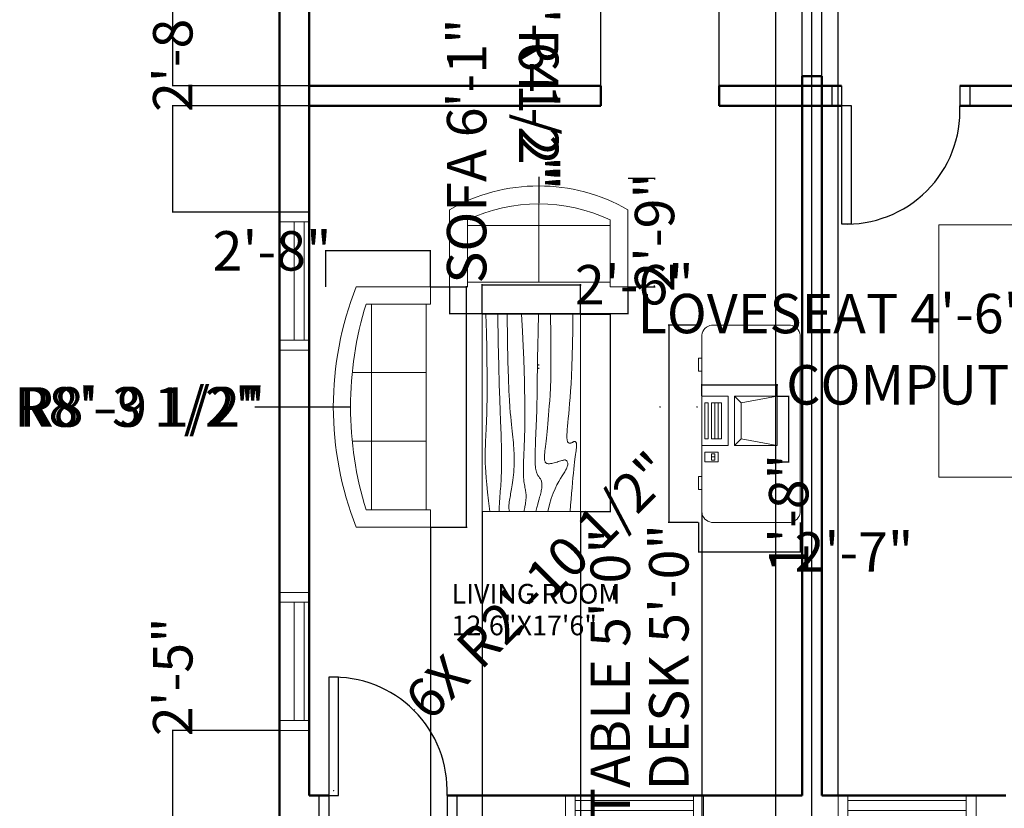
# Model space of a CAD drawing. Units: inches. Extents: x -51 to 1118, y -44 to 791.
# Tile 2 of 8: x -51 to 249, y 104 to 344. Entities that reach past the tile are written whole.
import ezdxf

# ---------------------------------------------------------------- set-up
doc = ezdxf.new("R2010")
doc.units = ezdxf.units.IN
doc.header["$MEASUREMENT"] = 0
for name, color, linetype, lineweight in [('A-ANNO-DIMS', 2, 'Continuous', 18), ('A-AREA-IDEN', 7, 'Continuous', 18), ('A-DOOR', 3, 'Continuous', 25), ('A-EQPM', 9, 'Continuous', 18), ('A-FURN', 8, 'Continuous', 18), ('A-GLAZ', 4, 'Continuous', 18), ('A-WALL', 7, 'Continuous', 50)]:
    doc.layers.add(name, color=color, linetype=linetype, lineweight=lineweight)
doc.styles.get("Standard").update_dxf_attribs({"font": 'arial.ttf'})
doc.dimstyles.get("Standard").update_dxf_attribs({"dimtxt": 12, "dimasz": 0.18, "dimexe": 0.18, "dimexo": 0.0625, "dimgap": 0.09, "dimtad": 0, "dimdec": 1, "dimzin": 0, "dimdsep": 46, "dimlunit": 3, "dimtxsty": 'Standard', "dimcen": 0.09, "dimadec": 0, "dimazin": 0, "dimtfac": 1, "dimtdec": 1, "dimtofl": 0, "dimtmove": 0, "dimatfit": 3, "dimfxl": 1, "dimtolj": 1, "dimtzin": 0, "dimarcsym": 0})

# ---------------------------------------------------------------- blocks, each defined once
blk = doc.blocks.new('Table - Rectangular Woodgrain 60 x 30 in.')
for p, q in [((0, 0), (0, -30)), ((60, 0), (0, 0)), ((60, -30), (60, 0)), ((0, -30), (60, -30))]:
    blk.add_line(p, q)
for points in [[(0, -2.4), (4.8155, -2.418), (9.0302, -2.4688), (12.709, -2.5477), (15.9167, -2.65), (18.7181, -2.7711), (21.1781, -2.9063), (23.3616, -3.0508), (25.3333, -3.2), (27.1477, -3.3495), (28.8172, -3.4958), (30.3437, -3.636), (31.7291, -3.7667), (32.9756, -3.8849), (34.0849, -3.9875), (35.059, -4.0714), (35.9, -4.1334), (36.6114, -4.1711), (37.2041, -4.1854), (37.6906, -4.1779), (38.0833, -4.15), (38.3948, -4.1034), (38.6375, -4.0396), (38.8239, -3.9602), (38.9666, -3.8667), (39.0764, -3.7608), (39.1573, -3.6448), (39.2116, -3.521), (39.2416, -3.3917), (39.2498, -3.2593), (39.2385, -3.1261), (39.21, -2.9944), (39.1666, -2.8667), (39.111, -2.7447), (39.0468, -2.6281), (38.978, -2.5163), (38.9083, -2.4083), (38.8418, -2.3035), (38.7823, -2.201), (38.7337, -2.1001), (38.7, -2), (38.6844, -1.9003), (38.6875, -1.8021), (38.7094, -1.707), (38.75, -1.6167), (38.8094, -1.5326), (38.8875, -1.4563), (38.9844, -1.3893), (39.1, -1.3333), (39.2351, -1.2896), (39.3937, -1.2583), (39.5804, -1.2396), (39.8, -1.2333), (40.057, -1.2396), (40.3562, -1.2583), (40.7023, -1.2896), (41.1, -1.3333), (41.5547, -1.3895), (42.0755, -1.4573), (42.6721, -1.5361), (43.3542, -1.625), (44.1316, -1.7233), (45.014, -1.8302), (46.0114, -1.9449), (47.1333, -2.0667), (48.3862, -2.1947), (49.7625, -2.3281), (51.2513, -2.4663), (52.8416, -2.6083), (54.5226, -2.7535), (56.2833, -2.9011), (58.1127, -3.0501), (60, -3.2)], [(0, -9.2), (6.5759, -9.0858), (11.9385, -9.0365), (16.2527, -9.0418), (19.6833, -9.0917), (22.3952, -9.1759), (24.5531, -9.2844), (26.322, -9.4069), (27.8666, -9.5333), (29.3241, -9.6553), (30.7203, -9.7719), (32.0532, -9.8837), (33.3208, -9.9917), (34.5213, -10.0965), (35.6526, -10.199), (36.7128, -10.2999), (37.7, -10.4), (38.6129, -10.4996), (39.4531, -10.5969), (40.223, -10.6895), (40.925, -10.775), (41.5613, -10.8512), (42.1344, -10.9156), (42.6465, -10.966), (43.1, -11), (43.4976, -11.0158), (43.8437, -11.0136), (44.143, -10.9942), (44.4, -10.9583), (44.6195, -10.9069), (44.8062, -10.8406), (44.9648, -10.7603), (45.1, -10.6667), (45.2155, -10.5598), (45.3114, -10.4365), (45.3871, -10.2929), (45.4416, -10.125), (45.4743, -9.929), (45.4844, -9.7011), (45.4709, -9.4371), (45.4333, -9.1333), (45.3716, -8.7883), (45.2896, -8.4104), (45.1919, -8.0107), (45.0833, -7.6), (44.9685, -7.1893), (44.8521, -6.7896), (44.7388, -6.4117), (44.6333, -6.0667), (44.54, -5.7628), (44.4614, -5.4979), (44.4001, -5.2675), (44.3583, -5.0667), (44.3384, -4.8909), (44.3427, -4.7354), (44.3736, -4.5956), (44.4333, -4.4667), (44.5236, -4.3453), (44.6427, -4.2333), (44.7884, -4.1339), (44.9583, -4.05), (45.1501, -3.9849), (45.3614, -3.9417), (45.59, -3.9234), (45.8333, -3.9333), (46.0915, -3.9749), (46.3734, -4.0531), (46.6906, -4.1736), (47.0542, -4.3417), (47.4756, -4.5629), (47.9661, -4.8427), (48.5372, -5.1866), (49.2, -5.6), (49.9676, -6.0844), (50.8594, -6.625), (51.8965, -7.2031), (53.1, -7.8), (54.491, -8.3969), (56.0906, -8.975), (57.9199, -9.5156), (60, -10)], [(0, -12.8), (5.1847, -12.9322), (9.6213, -13.0323), (13.3963, -13.1059), (16.5958, -13.1583), (19.3063, -13.1952), (21.614, -13.2219), (23.6054, -13.2439), (25.3666, -13.2667), (26.9728, -13.2947), (28.4531, -13.3281), (29.8256, -13.3663), (31.1083, -13.4083), (32.3191, -13.4535), (33.476, -13.501), (34.597, -13.5501), (35.7, -13.6), (36.7984, -13.6497), (37.8875, -13.6979), (38.9578, -13.743), (40, -13.7833), (41.0047, -13.8174), (41.9625, -13.8438), (42.864, -13.8607), (43.7, -13.8667), (44.4631, -13.8604), (45.1552, -13.8417), (45.7801, -13.8104), (46.3416, -13.7667), (46.8439, -13.7104), (47.2906, -13.6417), (47.6858, -13.5604), (48.0333, -13.4667), (48.3375, -13.3608), (48.6042, -13.2448), (48.8396, -13.121), (49.05, -12.9917), (49.2417, -12.8593), (49.4208, -12.7261), (49.5937, -12.5944), (49.7667, -12.4667), (49.9452, -12.3451), (50.1323, -12.2313), (50.3303, -12.1268), (50.5416, -12.0333), (50.7686, -11.9524), (51.0135, -11.8854), (51.2788, -11.8341), (51.5666, -11.8), (51.8785, -11.7843), (52.2116, -11.7865), (52.562, -11.8059), (52.926, -11.8417), (53.2998, -11.8931), (53.6795, -11.9594), (54.0614, -12.0397), (54.4416, -12.1333), (54.8223, -12.2401), (55.2293, -12.3625), (55.6942, -12.5037), (56.2489, -12.6667), (56.9251, -12.8547), (57.7545, -13.0708), (58.7689, -13.3182), (60, -13.6)], [(0, -18), (5.124, -17.7273), (9.6609, -17.5057), (13.6705, -17.3303), (17.2125, -17.1958), (20.3467, -17.0973), (23.1328, -17.0297), (25.6307, -16.9878), (27.9, -16.9667), (29.9928, -16.9617), (31.9302, -16.9703), (33.7254, -16.9907), (35.3917, -17.0208), (36.9423, -17.0588), (38.3906, -17.1026), (39.7499, -17.1503), (41.0333, -17.2), (42.2519, -17.2496), (43.4073, -17.2969), (44.4986, -17.3395), (45.525, -17.375), (46.4858, -17.4012), (47.3802, -17.4156), (48.2074, -17.416), (48.9667, -17.4), (49.6583, -17.3662), (50.2872, -17.3167), (50.8595, -17.2547), (51.3812, -17.1833), (51.8584, -17.1057), (52.2971, -17.025), (52.7034, -16.9443), (53.0833, -16.8667), (53.443, -16.7951), (53.789, -16.7313), (54.128, -16.6768), (54.4666, -16.6334), (54.8115, -16.6024), (55.1693, -16.5854), (55.5465, -16.5841), (55.95, -16.6), (56.3828, -16.6337), (56.8346, -16.6823), (57.2915, -16.7418), (57.7396, -16.8084), (58.165, -16.878), (58.5539, -16.9469), (58.8924, -17.0111), (59.1666, -17.0667), (59.3679, -17.1107), (59.5078, -17.1438), (59.6032, -17.1675), (59.6708, -17.1833), (59.7275, -17.193), (59.7901, -17.1979), (59.8753, -17.1998), (60, -17.2)], [(0, -22.4), (8.0098, -22.2501), (14.4094, -22.1011), (19.4168, -21.9535), (23.25, -21.8083), (26.1269, -21.6663), (28.2656, -21.5281), (29.884, -21.3947), (31.2, -21.2667), (32.3967, -21.1448), (33.5172, -21.0292), (34.5697, -20.9198), (35.5625, -20.8167), (36.5037, -20.7198), (37.4015, -20.6292), (38.2642, -20.5448), (39.1, -20.4667), (39.9164, -20.3951), (40.7187, -20.3313), (41.5117, -20.2768), (42.3, -20.2333), (43.0883, -20.2024), (43.8812, -20.1854), (44.6836, -20.1841), (45.5, -20.2), (46.3328, -20.234), (47.1747, -20.2844), (48.0163, -20.3488), (48.8479, -20.425), (49.66, -20.5106), (50.4429, -20.6031), (51.1872, -20.7004), (51.8833, -20.8), (52.5246, -20.8999), (53.1166, -20.9995), (53.6681, -21.0983), (54.1875, -21.1958), (54.6834, -21.2919), (55.1646, -21.3859), (55.6394, -21.4777), (56.1167, -21.5667), (56.6028, -21.6515), (57.0961, -21.7266), (57.5929, -21.7852), (58.0896, -21.8208), (58.5823, -21.8268), (59.0674, -21.7964), (59.5412, -21.723), (60, -21.6)], [(0, -25.2), (8.6355, -25.0504), (15.7026, -24.9031), (21.4049, -24.7606), (25.9458, -24.625), (29.529, -24.4988), (32.3578, -24.3844), (34.6359, -24.284), (36.5667, -24.2), (38.3213, -24.1341), (39.9417, -24.0854), (41.437, -24.0523), (42.8167, -24.0333), (44.0901, -24.0268), (45.2667, -24.0313), (46.3557, -24.0451), (47.3667, -24.0667), (48.309, -24.0947), (49.1928, -24.1287), (50.0284, -24.168), (50.826, -24.2125), (51.5959, -24.2617), (52.3483, -24.3151), (53.0935, -24.3725), (53.8417, -24.4334), (54.6009, -24.497), (55.3699, -24.561), (56.1454, -24.6226), (56.9239, -24.6792), (57.7021, -24.7279), (58.4764, -24.7662), (59.2435, -24.7911), (60, -24.8)], [(0, -28.8), (5.6867, -28.6681), (10.45, -28.5698), (14.407, -28.5012), (17.675, -28.4584), (20.3711, -28.4374), (22.6125, -28.4344), (24.5164, -28.4455), (26.2, -28.4667), (27.762, -28.4947), (29.2276, -28.5281), (30.6033, -28.5663), (31.8958, -28.6084), (33.1118, -28.6535), (34.2578, -28.7011), (35.3405, -28.7501), (36.3666, -28.8), (37.3443, -28.8497), (38.288, -28.8974), (39.2137, -28.9412), (40.1375, -28.9792), (41.0753, -29.0093), (42.0432, -29.0297), (43.0572, -29.0384), (44.1333, -29.0333), (45.2936, -29.0114), (46.5843, -28.9641), (48.0579, -28.8816), (49.7666, -28.7542), (51.7629, -28.5721), (54.0989, -28.3255), (56.8272, -28.0048), (60, -27.6)]]:
    blk.add_lwpolyline(points)
blk = doc.blocks.new('Computer Terminal')
for p, q in [((-10, 11.5), (5, 11.5)), ((-8, 0.5), (-10, 11.5)), ((-10, -1.5), (-10, 11.5)), ((5, 11.5), (3, 0.5)), ((5, 11.5), (5, -1.5)), ((-10, -1.5), (-8, 0.5)), ((3, 0.5), (-8, 0.5)), ((3, 0.5), (5, -1.5)), ((5, -1.5), (-10, -1.5)), ((-10, -11.5), (-10, -3.5)), ((-10, -3.5), (5, -3.5)), ((-8, -5.5), (-8, -8.5)), ((3, -5.5), (-8, -5.5)), ((3, -8.5), (3, -5.5)), ((5, -3.5), (5, -11.5)), ((3, -6.5), (-8, -6.5)), ((-8, -7.5), (3, -7.5)), ((-8, -8.5), (3, -8.5)), ((10, -6.5), (7, -6.5)), ((7, -6.5), (7, -10.5)), ((9.5, -7.5), (7.5, -7.5)), ((7.5, -7.5), (7.5, -8.5)), ((7.5, -8.5), (9.5, -8.5)), ((8.5, -7.5), (8.5, -8.5)), ((9.5, -8.5), (9.5, -7.5)), ((10, -10.5), (10, -6.5)), ((5, -11.5), (-10, -11.5)), ((-8, -9.5), (-8, -10.5)), ((3, -9.5), (-8, -9.5)), ((-8, -10.5), (3, -10.5)), ((3, -10.5), (3, -9.5)), ((7, -10.5), (10, -10.5))]:
    blk.add_line(p, q)
blk = doc.blocks.new('Desk - 30 x 60 in.')
for p, q in [((-26.999995, 0), (26.999995, 0)), ((-29.999995, -27), (-29.999995, -3)), ((29.999995, -3), (29.999995, -27)), ((26.999995, -30), (-26.999995, -30)), ((-20.000005, -30), (-20.000005, -31)), ((-20.000005, -31), (-16.000005, -31)), ((-16.000005, -31), (-16.000005, -30)), ((15.999995, -31), (15.999995, -30)), ((19.999995, -31), (15.999995, -31)), ((19.999995, -30), (19.999995, -31))]:
    blk.add_line(p, q)
for centre, start, end in [((-26.499995, -3.5), 98.1301, 171.8699), ((26.499995, -3.5), 8.130102, 81.8699), ((-26.499995, -26.5), 188.1301, 261.8699), ((26.499995, -26.5), 278.1301, 351.8699)]:
    blk.add_arc(centre, 3.535534, start, end)
blk = doc.blocks.new('Bed - Queen')
for p, q in [((0, -80.00003), (0, 0)), ((0, 0), (59.99999, 0)), ((59.99999, 0), (59.99999, -80.00003)), ((7.99999, -1.2), (28.79998, -1.2)), ((7.99999, -14.4), (7.99999, -1.2)), ((28.79998, -1.2), (28.79998, -14.4)), ((31.19999, -1.2), (51.99999, -1.2)), ((31.19999, -14.4), (31.19999, -1.2)), ((51.99999, -1.2), (51.99999, -16.4)), ((0, -14.4), (44.8, -14.4)), ((59.99999, -29.6), (44.8, -14.4)), ((44.8, -14.4), (44.8, -29.6)), ((44.8, -16.8), (0, -16.8)), ((51.99999, -16.4), (46.79936, -16.4)), ((44.8, -29.6), (59.99999, -29.6)), ((59.99999, -80.00003), (0, -80.00003))]:
    blk.add_line(p, q)
blk = doc.blocks.new('Sofa - Roundback Loveseat 5 ft.')
for p, q in [((0, -32.44198), (0, -5.99998)), ((-24, -33.99998), (-24, -11.46958)), ((24.00004, -33.99998), (24.00004, -11.46958)), ((-23.9998, -13.38178), (23.99986, -13.38178)), ((-24, -32.44198), (24.00004, -32.44198))]:
    blk.add_line(p, q)
for points in [[(-24, -33.99998), (-30, -33.99998), (-30, -7.99998)], [(30.00004, -7.99998), (30.00004, -33.99998), (24.00004, -33.99998)]]:
    blk.add_lwpolyline(points)
for centre, radius, start, end in [((0, -60.24998), 60.24998, 60.13715, 119.8628), ((0, -61.38438), 55.38444, 64.32083, 115.6792)]:
    blk.add_arc(centre, radius, start, end)
blk = doc.blocks.new('Sofa - Roundback 7 ft.')
for p, q in [((-12.00002, -32.4421), (-12.00003, -6.5971)), ((11.99997, -32.4421), (11.99998, -6.5971)), ((-36.000027, -34), (-36.000027, -11.4696)), ((-35.999844, -13.3819), (35.9998, -13.3819)), ((35.99998, -34), (35.99998, -11.4696)), ((-36.000027, -32.4421), (35.99998, -32.4421))]:
    blk.add_line(p, q)
for points in [[(-36.000027, -34), (-42.000027, -34), (-42.000027, -8)], [(41.99998, -8), (41.99998, -34), (35.99998, -34)]]:
    blk.add_lwpolyline(points)
for centre, radius, start, end in [((0, -114.25), 114.25, 68.43141, 111.5686), ((-0.00001, -127.1968), 121.1968, 72.72033, 107.2797)]:
    blk.add_arc(centre, radius, start, end)
blk = doc.blocks.new('WIN-36IN')
for p, q in [((9, 42), (0, 42)), ((9, 39), (0, 39)), ((0, 39), (0, 3)), ((4.5, 3), (4.5, 39)), ((7.5, 3), (7.5, 39)), ((9, 3), (9, 39)), ((0, 3), (9, 3)), ((0, 0), (9, 0))]:
    blk.add_line(p, q)
blk = doc.blocks.new('DOOR-36IN-FRAME-9IN')
for p, q in [((0, 36.03), (0, 45.03)), ((3, 36.03), (3, 45.03)), ((39, 36.03), (39, 45.03)), ((42, 36.03), (42, 45.03))]:
    blk.add_line(p, q)
blk.add_lwpolyline([(39, 36.03), (36, 36.03), (36, 0.03), (39, 0.03)], close=True)
blk.add_arc((37.5, 34.53), 34.53, 177.5104, 272.4896)
blk = doc.blocks.new('DOOR-36IN-FRAME-6IN')
for p, q in [((0, 42), (6, 42)), ((0, 39), (6, 39)), ((0, 3), (6, 3)), ((0, 0), (6, 0))]:
    blk.add_line(p, q)
blk.add_lwpolyline([(6, 3), (42, 3), (42, 6), (6, 6)], close=True)
blk.add_arc((7.5, 4.5), 34.53, 357.5104, 92.4896)
blk = doc.blocks.new('*D28')
at = {"layer": 'A-ANNO-DIMS', "color": 0, "lineweight": -2, "transparency": 16777216}
for p, q in [((119.72, 254.44), (128.83, 254.44)), ((128.65, 254.26), (128.65, 194.62)), ((119.72, 194.44), (128.83, 194.44)), ((128.65, 194.44), (128.65, 194.26))]:
    blk.add_line(p, q, dxfattribs=at)
at = {"layer": 'A-ANNO-DIMS', "color": 0, "transparency": 16777216}
for points in [[(128.62, 254.26), (128.68, 254.26), (128.65, 254.44)], [(128.62, 194.62), (128.68, 194.62), (128.65, 194.44)]]:
    blk.add_solid(points, dxfattribs=at)
at = {"layer": 'Defpoints', "color": 0, "transparency": 16777216}
for p in [(119.65, 254.44), (119.65, 194.44), (128.65, 194.44)]:
    blk.add_point(p, dxfattribs=at)
at = {"layer": 'A-ANNO-DIMS', "color": 0, "transparency": 16777216, "insert": (128.65, 113.08), "char_height": 12, "attachment_point": 5, "rotation": 90}
blk.add_mtext('\\A1;COFFEE TABLE 5\'-0"', dxfattribs=at)
blk = doc.blocks.new('*D29')
at = {"layer": 'A-ANNO-DIMS', "color": 0, "lineweight": -2, "transparency": 16777216}
for p, q in [((89.65, 254.5), (89.65, 263.62)), ((119.65, 254.5), (119.65, 263.62)), ((89.83, 263.44), (119.47, 263.44)), ((119.65, 263.44), (119.83, 263.44))]:
    blk.add_line(p, q, dxfattribs=at)
at = {"layer": 'A-ANNO-DIMS', "color": 0, "transparency": 16777216}
for points in [[(89.83, 263.47), (89.83, 263.41), (89.65, 263.44)], [(119.47, 263.47), (119.47, 263.41), (119.65, 263.44)]]:
    blk.add_solid(points, dxfattribs=at)
at = {"layer": 'Defpoints', "color": 0, "transparency": 16777216}
for p in [(119.65, 263.44), (89.65, 254.44), (119.65, 254.44)]:
    blk.add_point(p, dxfattribs=at)
at = {"layer": 'A-ANNO-DIMS', "color": 0, "transparency": 16777216, "insert": (135.98, 263.44), "char_height": 12, "attachment_point": 5}
blk.add_mtext('\\A1;2\'-6"', dxfattribs=at)
blk = doc.blocks.new('*D30')
at = {"layer": 'A-ANNO-DIMS', "color": 0, "lineweight": -2, "transparency": 16777216}
for p, q in [((156.48, 229.58), (156.48, 233.14)), ((156.66, 232.96), (179.3, 232.96)), ((179.48, 229.58), (179.48, 233.14)), ((179.48, 232.96), (179.66, 232.96))]:
    blk.add_line(p, q, dxfattribs=at)
at = {"layer": 'A-ANNO-DIMS', "color": 0, "transparency": 16777216}
for points in [[(156.66, 232.99), (156.66, 232.93), (156.48, 232.96)], [(179.3, 232.99), (179.3, 232.93), (179.48, 232.96)]]:
    blk.add_solid(points, dxfattribs=at)
at = {"layer": 'Defpoints', "color": 0, "transparency": 16777216}
for p in [(179.48, 232.96), (156.48, 229.51), (179.48, 229.51)]:
    blk.add_point(p, dxfattribs=at)
at = {"layer": 'A-ANNO-DIMS', "color": 0, "transparency": 16777216, "insert": (250.58, 232.96), "char_height": 12, "attachment_point": 5}
blk.add_mtext('\\A1;COMPUTER 1\'-11"', dxfattribs=at)
blk = doc.blocks.new('*D31')
at = {"layer": 'A-ANNO-DIMS', "color": 0, "lineweight": -2, "transparency": 16777216}
for p, q in [((179.54, 229.51), (183.11, 229.51)), ((182.93, 229.33), (182.93, 209.69)), ((179.54, 209.51), (183.11, 209.51)), ((182.93, 209.51), (182.93, 209.33))]:
    blk.add_line(p, q, dxfattribs=at)
at = {"layer": 'A-ANNO-DIMS', "color": 0, "transparency": 16777216}
for points in [[(182.9, 229.33), (182.96, 229.33), (182.93, 229.51)], [(182.9, 209.69), (182.96, 209.69), (182.93, 209.51)]]:
    blk.add_solid(points, dxfattribs=at)
at = {"layer": 'Defpoints', "color": 0, "transparency": 16777216}
for p in [(179.48, 229.51), (179.48, 209.51), (182.93, 209.51)]:
    blk.add_point(p, dxfattribs=at)
at = {"layer": 'A-ANNO-DIMS', "color": 0, "transparency": 16777216, "insert": (182.93, 193.86), "char_height": 12, "attachment_point": 5, "rotation": 90}
blk.add_mtext('\\A1;1\'-8"', dxfattribs=at)
blk = doc.blocks.new('*D32')
at = {"layer": 'A-ANNO-DIMS', "color": 0, "lineweight": -2, "transparency": 16777216}
for p, q in [((155.41, 251.11), (146.3, 251.11)), ((146.48, 250.93), (146.48, 191.29)), ((155.41, 191.11), (146.3, 191.11)), ((146.48, 191.11), (146.48, 190.93))]:
    blk.add_line(p, q, dxfattribs=at)
at = {"layer": 'A-ANNO-DIMS', "color": 0, "transparency": 16777216}
for points in [[(146.45, 250.93), (146.51, 250.93), (146.48, 251.11)], [(146.45, 191.29), (146.51, 191.29), (146.48, 191.11)]]:
    blk.add_solid(points, dxfattribs=at)
at = {"layer": 'Defpoints', "color": 0, "transparency": 16777216}
for p in [(155.48, 251.11), (146.48, 191.11), (155.48, 191.11)]:
    blk.add_point(p, dxfattribs=at)
at = {"layer": 'A-ANNO-DIMS', "color": 0, "transparency": 16777216, "insert": (146.48, 150.04), "char_height": 12, "attachment_point": 5, "rotation": 90}
blk.add_mtext('\\A1;DESK 5\'-0"', dxfattribs=at)
blk = doc.blocks.new('*D33')
at = {"layer": 'A-ANNO-DIMS', "color": 0, "lineweight": -2, "transparency": 16777216}
for p, q in [((155.48, 191.05), (155.48, 181.93)), ((186.48, 191.05), (186.48, 181.93)), ((155.66, 182.11), (186.3, 182.11)), ((186.48, 182.11), (186.66, 182.11))]:
    blk.add_line(p, q, dxfattribs=at)
at = {"layer": 'A-ANNO-DIMS', "color": 0, "transparency": 16777216}
for points in [[(155.66, 182.14), (155.66, 182.08), (155.48, 182.11)], [(186.3, 182.14), (186.3, 182.08), (186.48, 182.11)]]:
    blk.add_solid(points, dxfattribs=at)
at = {"layer": 'Defpoints', "color": 0, "transparency": 16777216}
for p in [(155.48, 191.11), (186.48, 191.11), (186.48, 182.11)]:
    blk.add_point(p, dxfattribs=at)
at = {"layer": 'A-ANNO-DIMS', "color": 0, "transparency": 16777216, "insert": (202.8, 182.11), "char_height": 12, "attachment_point": 5}
blk.add_mtext('\\A1;2\'-7"', dxfattribs=at)
blk = doc.blocks.new('*D36')
at = {"layer": 'A-ANNO-DIMS', "color": 0, "lineweight": -2, "transparency": 16777216}
for p, q in [((79.8, 262.73), (79.8, 254.48)), ((134, 262.73), (134, 254.48)), ((79.98, 254.66), (133.82, 254.66)), ((134, 254.66), (134.18, 254.66))]:
    blk.add_line(p, q, dxfattribs=at)
at = {"layer": 'A-ANNO-DIMS', "color": 0, "transparency": 16777216}
for points in [[(79.98, 254.69), (79.98, 254.63), (79.8, 254.66)], [(133.82, 254.69), (133.82, 254.63), (134, 254.66)]]:
    blk.add_solid(points, dxfattribs=at)
at = {"layer": 'Defpoints', "color": 0, "transparency": 16777216}
for p in [(79.8, 262.79), (134, 262.79), (134, 254.66)]:
    blk.add_point(p, dxfattribs=at)
at = {"layer": 'A-ANNO-DIMS', "color": 0, "transparency": 16777216, "insert": (196.54, 254.66), "char_height": 12, "attachment_point": 5}
blk.add_mtext('\\A1;LOVESEAT 4\'-6"', dxfattribs=at)
blk = doc.blocks.new('*D37')
at = {"layer": 'A-ANNO-DIMS', "color": 0, "lineweight": -2, "transparency": 16777216}
for p, q in [((134.06, 295.91), (142.31, 295.91)), ((142.13, 295.73), (142.13, 295.49)), ((134.06, 262.79), (142.31, 262.79)), ((142.13, 262.97), (142.13, 263.21))]:
    blk.add_line(p, q, dxfattribs=at)
at = {"layer": 'A-ANNO-DIMS', "color": 0, "transparency": 16777216}
for points in [[(142.1, 295.73), (142.16, 295.73), (142.13, 295.91)], [(142.1, 262.97), (142.16, 262.97), (142.13, 262.79)]]:
    blk.add_solid(points, dxfattribs=at)
at = {"layer": 'Defpoints', "color": 0, "transparency": 16777216}
for p in [(134, 295.91), (142.13, 295.91), (134, 262.79)]:
    blk.add_point(p, dxfattribs=at)
at = {"layer": 'A-ANNO-DIMS', "color": 0, "transparency": 16777216, "insert": (142.13, 279.35), "char_height": 12, "attachment_point": 5, "rotation": 90}
blk.add_mtext('\\A1;2\'-9"', dxfattribs=at)
blk = doc.blocks.new('*D38')
at = {"layer": 'A-ANNO-DIMS', "color": 0, "lineweight": -2, "transparency": 16777216}
for p, q in [((74.06, 262.79), (85.15, 262.79)), ((84.97, 262.79), (84.97, 262.97)), ((84.97, 189.87), (84.97, 262.61)), ((74.06, 189.69), (85.15, 189.69))]:
    blk.add_line(p, q, dxfattribs=at)
at = {"layer": 'A-ANNO-DIMS', "color": 0, "transparency": 16777216}
for points in [[(84.94, 262.61), (85, 262.61), (84.97, 262.79)], [(84.94, 189.87), (85, 189.87), (84.97, 189.69)]]:
    blk.add_solid(points, dxfattribs=at)
at = {"layer": 'Defpoints', "color": 0, "transparency": 16777216}
for p in [(74, 262.79), (84.97, 262.79), (74, 189.69)]:
    blk.add_point(p, dxfattribs=at)
at = {"layer": 'A-ANNO-DIMS', "color": 0, "transparency": 16777216, "insert": (84.97, 304.13), "char_height": 12, "attachment_point": 5, "rotation": 90}
blk.add_mtext('\\A1;SOFA 6\'-1"', dxfattribs=at)
blk = doc.blocks.new('*D39')
at = {"layer": 'A-ANNO-DIMS', "color": 0, "lineweight": -2, "transparency": 16777216}
for p, q in [((42.09, 273.75), (41.91, 273.75)), ((42.09, 262.85), (42.09, 273.93)), ((73.82, 273.75), (42.27, 273.75)), ((74, 262.85), (74, 273.93))]:
    blk.add_line(p, q, dxfattribs=at)
at = {"layer": 'A-ANNO-DIMS', "color": 0, "transparency": 16777216}
for points in [[(42.27, 273.78), (42.27, 273.72), (42.09, 273.75)], [(73.82, 273.78), (73.82, 273.72), (74, 273.75)]]:
    blk.add_solid(points, dxfattribs=at)
at = {"layer": 'Defpoints', "color": 0, "transparency": 16777216}
for p in [(42.09, 273.75), (42.09, 262.79), (74, 262.79)]:
    blk.add_point(p, dxfattribs=at)
at = {"layer": 'A-ANNO-DIMS', "color": 0, "transparency": 16777216, "insert": (25.77, 273.75), "char_height": 12, "attachment_point": 5}
blk.add_mtext('\\A1;2\'-8"', dxfattribs=at)
blk = doc.blocks.new('*D44')
at = {"layer": 'A-ANNO-DIMS', "color": 0, "lineweight": -2, "transparency": 16777216}
for p, q in [((27.96, 127.77), (-4.61, 127.77)), ((-4.43, 127.77), (-4.43, 127.95)), ((-4.43, 99.12), (-4.43, 127.59)), ((36.96, 98.94), (-4.61, 98.94))]:
    blk.add_line(p, q, dxfattribs=at)
at = {"layer": 'A-ANNO-DIMS', "color": 0, "transparency": 16777216}
for points in [[(-4.46, 127.59), (-4.4, 127.59), (-4.43, 127.77)], [(-4.46, 99.12), (-4.4, 99.12), (-4.43, 98.94)]]:
    blk.add_solid(points, dxfattribs=at)
at = {"layer": 'Defpoints', "color": 0, "transparency": 16777216}
for p in [(-4.43, 127.77), (28.02, 127.77), (37.02, 98.94)]:
    blk.add_point(p, dxfattribs=at)
at = {"layer": 'A-ANNO-DIMS', "color": 0, "transparency": 16777216, "insert": (-4.43, 144.09), "char_height": 12, "attachment_point": 5, "rotation": 90}
blk.add_mtext('\\A1;2\'-5"', dxfattribs=at)
blk = doc.blocks.new('*D45')
at = {"layer": 'A-ANNO-DIMS', "color": 0, "lineweight": -2, "transparency": 16777216}
for p, q in [((36.96, 317.94), (-4.61, 317.94)), ((-4.43, 317.94), (-4.43, 318.12)), ((-4.43, 285.72), (-4.43, 317.76)), ((36.96, 285.54), (-4.61, 285.54))]:
    blk.add_line(p, q, dxfattribs=at)
at = {"layer": 'A-ANNO-DIMS', "color": 0, "transparency": 16777216}
for points in [[(-4.46, 317.76), (-4.4, 317.76), (-4.43, 317.94)], [(-4.46, 285.72), (-4.4, 285.72), (-4.43, 285.54)]]:
    blk.add_solid(points, dxfattribs=at)
at = {"layer": 'Defpoints', "color": 0, "transparency": 16777216}
for p in [(-4.43, 317.94), (37.02, 317.94), (37.02, 285.54)]:
    blk.add_point(p, dxfattribs=at)
at = {"layer": 'A-ANNO-DIMS', "color": 0, "transparency": 16777216, "insert": (-4.43, 348.24), "char_height": 12, "attachment_point": 5, "rotation": 90}
blk.add_mtext('\\A1;2\'-8 1/2"', dxfattribs=at)
blk = doc.blocks.new('*D46')
at = {"layer": 'A-ANNO-DIMS', "color": 0, "lineweight": -2, "transparency": 16777216}
for p, q in [((36.96, 375.28), (-4.61, 375.28)), ((-4.43, 375.28), (-4.43, 375.46)), ((-4.43, 324.12), (-4.43, 375.1)), ((36.96, 323.94), (-4.61, 323.94))]:
    blk.add_line(p, q, dxfattribs=at)
at = {"layer": 'A-ANNO-DIMS', "color": 0, "transparency": 16777216}
for points in [[(-4.46, 375.1), (-4.4, 375.1), (-4.43, 375.28)], [(-4.46, 324.12), (-4.4, 324.12), (-4.43, 323.94)]]:
    blk.add_solid(points, dxfattribs=at)
at = {"layer": 'Defpoints', "color": 0, "transparency": 16777216}
for p in [(-4.43, 375.28), (37.02, 375.28), (37.02, 323.94)]:
    blk.add_point(p, dxfattribs=at)
at = {"layer": 'A-ANNO-DIMS', "color": 0, "transparency": 16777216, "insert": (-4.43, 405.72), "char_height": 12, "attachment_point": 5, "rotation": 90}
blk.add_mtext('\\A1;4\'-3 1/2"', dxfattribs=at)
blk = doc.blocks.new('*D55')
at = {"layer": 'A-ANNO-DIMS', "color": 0, "lineweight": -2, "transparency": 16777216}
for p, q in [((193.02, 108), (193.02, 638.57)), ((193.2, 638.39), (197.79, 638.39)), ((197.97, 108), (197.97, 638.57)), ((197.97, 638.39), (198.15, 638.39))]:
    blk.add_line(p, q, dxfattribs=at)
at = {"layer": 'A-ANNO-DIMS', "color": 0, "transparency": 16777216}
for points in [[(193.2, 638.42), (193.2, 638.36), (193.02, 638.39)], [(197.79, 638.42), (197.79, 638.36), (197.97, 638.39)]]:
    blk.add_solid(points, dxfattribs=at)
at = {"layer": 'Defpoints', "color": 0, "transparency": 16777216}
for p in [(197.97, 638.39), (193.02, 107.94), (197.97, 107.94)]:
    blk.add_point(p, dxfattribs=at)
at = {"layer": 'A-ANNO-DIMS', "color": 0, "transparency": 16777216, "insert": (214.19, 638.39), "char_height": 12, "attachment_point": 5}
blk.add_mtext('\\A1;0\'-5"', dxfattribs=at)
blk = doc.blocks.new('*D57')
at = {"layer": 'A-ANNO-DIMS', "color": 0, "lineweight": -2, "transparency": 16777216}
for p, q in [((179.02, 57), (179.02, 638.57)), ((179.2, 638.39), (189.84, 638.39)), ((190.02, 57), (190.02, 638.57)), ((190.02, 638.39), (190.2, 638.39))]:
    blk.add_line(p, q, dxfattribs=at)
at = {"layer": 'A-ANNO-DIMS', "color": 0, "transparency": 16777216}
for points in [[(179.2, 638.42), (179.2, 638.36), (179.02, 638.39)], [(189.84, 638.42), (189.84, 638.36), (190.02, 638.39)]]:
    blk.add_solid(points, dxfattribs=at)
at = {"layer": 'Defpoints', "color": 0, "transparency": 16777216}
for p in [(190.02, 638.39), (179.02, 56.94), (190.02, 56.94)]:
    blk.add_point(p, dxfattribs=at)
at = {"layer": 'A-ANNO-DIMS', "color": 0, "transparency": 16777216, "insert": (210.9, 638.39), "char_height": 12, "attachment_point": 5}
blk.add_mtext('\\A1;0\'-11"', dxfattribs=at)
blk = doc.blocks.new('*D59')
at = {"layer": 'A-ANNO-DIMS', "color": 0, "lineweight": -2, "transparency": 16777216}
for p, q in [((89.65, 194.38), (89.65, -26.69)), ((74, 189.63), (74, -26.69)), ((74.18, -26.51), (89.47, -26.51)), ((89.65, -26.51), (89.83, -26.51))]:
    blk.add_line(p, q, dxfattribs=at)
at = {"layer": 'A-ANNO-DIMS', "color": 0, "transparency": 16777216}
for points in [[(74.18, -26.48), (74.18, -26.54), (74, -26.51)], [(89.47, -26.48), (89.47, -26.54), (89.65, -26.51)]]:
    blk.add_solid(points, dxfattribs=at)
at = {"layer": 'Defpoints', "color": 0, "transparency": 16777216}
for p in [(89.65, 194.44), (74, 189.69), (89.65, -26.51)]:
    blk.add_point(p, dxfattribs=at)
at = {"layer": 'A-ANNO-DIMS', "color": 0, "transparency": 16777216, "insert": (119.29, -26.51), "char_height": 12, "attachment_point": 5}
blk.add_mtext('\\A1;1\'-3 1/2"', dxfattribs=at)
blk = doc.blocks.new('*D60')
at = {"layer": 'A-ANNO-DIMS', "color": 0, "lineweight": -2, "transparency": 16777216}
for p, q in [((119.65, 194.38), (119.65, -26.69)), ((156.48, 194.05), (156.48, -26.69)), ((119.83, -26.51), (122.03, -26.51)), ((156.3, -26.51), (154.1, -26.51))]:
    blk.add_line(p, q, dxfattribs=at)
at = {"layer": 'A-ANNO-DIMS', "color": 0, "transparency": 16777216}
for points in [[(119.83, -26.48), (119.83, -26.54), (119.65, -26.51)], [(156.3, -26.48), (156.3, -26.54), (156.48, -26.51)]]:
    blk.add_solid(points, dxfattribs=at)
at = {"layer": 'Defpoints', "color": 0, "transparency": 16777216}
for p in [(119.65, 194.44), (156.48, 194.11), (156.48, -26.51)]:
    blk.add_point(p, dxfattribs=at)
at = {"layer": 'A-ANNO-DIMS', "color": 0, "transparency": 16777216, "insert": (138.06, -26.51), "char_height": 12, "attachment_point": 5}
blk.add_mtext('\\A1;3\'-1"', dxfattribs=at)
blk = doc.blocks.new('*D61')
at = {"layer": 'A-ANNO-DIMS', "color": 0, "lineweight": -2, "transparency": 16777216}
for p, q in [((125.75, 324), (125.75, 638.57)), ((125.93, 638.39), (127.71, 638.39)), ((161.57, 638.39), (159.79, 638.39)), ((161.75, 324), (161.75, 638.57))]:
    blk.add_line(p, q, dxfattribs=at)
at = {"layer": 'A-ANNO-DIMS', "color": 0, "transparency": 16777216}
for points in [[(125.93, 638.42), (125.93, 638.36), (125.75, 638.39)], [(161.57, 638.42), (161.57, 638.36), (161.75, 638.39)]]:
    blk.add_solid(points, dxfattribs=at)
at = {"layer": 'Defpoints', "color": 0, "transparency": 16777216}
for p in [(161.75, 638.39), (125.75, 323.94), (161.75, 323.94)]:
    blk.add_point(p, dxfattribs=at)
at = {"layer": 'A-ANNO-DIMS', "color": 0, "transparency": 16777216, "insert": (143.75, 638.39), "char_height": 12, "attachment_point": 5}
blk.add_mtext('\\A1;3\'-0"', dxfattribs=at)
blk = doc.blocks.new('*D62')
at = {"layer": 'A-ANNO-DIMS', "color": 0, "lineweight": -2, "transparency": 16777216}
for p, q in [((161.75, 324), (161.75, 638.57)), ((161.93, 638.39), (186.84, 638.39)), ((187.02, 327), (187.02, 638.57)), ((187.02, 638.39), (187.2, 638.39))]:
    blk.add_line(p, q, dxfattribs=at)
at = {"layer": 'A-ANNO-DIMS', "color": 0, "transparency": 16777216}
for points in [[(161.93, 638.42), (161.93, 638.36), (161.75, 638.39)], [(186.84, 638.42), (186.84, 638.36), (187.02, 638.39)]]:
    blk.add_solid(points, dxfattribs=at)
at = {"layer": 'Defpoints', "color": 0, "transparency": 16777216}
for p in [(187.02, 638.39), (187.02, 326.94), (161.75, 323.94)]:
    blk.add_point(p, dxfattribs=at)
at = {"layer": 'A-ANNO-DIMS', "color": 0, "transparency": 16777216, "insert": (217.32, 638.39), "char_height": 12, "attachment_point": 5}
blk.add_mtext('\\A1;2\'-1 1/2"', dxfattribs=at)
blk = doc.blocks.new('*D67')
at = {"layer": 'A-ANNO-DIMS', "color": 0, "lineweight": -2, "transparency": 16777216}
for p, q in [((69.19, 134.11), (69.07, 133.99)), ((44.43, 109.44), (44.61, 109.44)), ((44.52, 109.35), (44.52, 109.53))]:
    blk.add_line(p, q, dxfattribs=at)
at = {"layer": 'A-ANNO-DIMS', "color": 0, "transparency": 16777216}
blk.add_solid([(69.05, 134.01), (69.09, 133.96), (68.94, 133.86)], dxfattribs=at)
at = {"layer": 'Defpoints', "color": 0, "transparency": 16777216}
for p in [(68.94, 133.86), (44.52, 109.44)]:
    blk.add_point(p, dxfattribs=at)
at = {"layer": 'A-ANNO-DIMS', "color": 0, "transparency": 16777216, "insert": (106.92, 171.84), "char_height": 12, "attachment_point": 5, "rotation": 45.0005}
blk.add_mtext('\\A1;6X R2\'-10 1/2"', dxfattribs=at)
blk = doc.blocks.new('*D68')
at = {"layer": 'A-ANNO-DIMS', "color": 0, "lineweight": -2, "transparency": 16777216}
for p, q in [((22.11, 226.24), (49.45, 226.24)), ((155.02, 226.24), (155.2, 226.24)), ((155.11, 226.15), (155.11, 226.33))]:
    blk.add_line(p, q, dxfattribs=at)
at = {"layer": 'A-ANNO-DIMS', "color": 0, "transparency": 16777216}
blk.add_solid([(49.45, 226.27), (49.45, 226.21), (49.63, 226.24)], dxfattribs=at)
at = {"layer": 'Defpoints', "color": 0, "transparency": 16777216}
for p in [(49.63, 226.24), (155.11, 226.24)]:
    blk.add_point(p, dxfattribs=at)
at = {"layer": 'A-ANNO-DIMS', "color": 0, "transparency": 16777216, "insert": (-13.65, 226.24), "char_height": 12, "attachment_point": 5, "rotation": 359.9999}
blk.add_mtext('\\A1;R8\'-9 1/2"', dxfattribs=at)
blk = doc.blocks.new('*D69')
at = {"layer": 'A-ANNO-DIMS', "color": 0, "lineweight": -2, "transparency": 16777216}
for p, q in [((20.52, 226.24), (44.23, 226.24)), ((143.75, 226.24), (143.93, 226.24)), ((143.84, 226.15), (143.84, 226.33))]:
    blk.add_line(p, q, dxfattribs=at)
at = {"layer": 'A-ANNO-DIMS', "color": 0, "transparency": 16777216}
blk.add_solid([(44.23, 226.27), (44.23, 226.21), (44.41, 226.24)], dxfattribs=at)
at = {"layer": 'Defpoints', "color": 0, "transparency": 16777216}
for p in [(44.41, 226.24), (143.84, 226.24)]:
    blk.add_point(p, dxfattribs=at)
at = {"layer": 'A-ANNO-DIMS', "color": 0, "transparency": 16777216, "insert": (-15.24, 226.24), "char_height": 12, "attachment_point": 5, "rotation": 359.9998}
blk.add_mtext('\\A1;R8\'-3 1/2"', dxfattribs=at)
blk = doc.blocks.new('*D70')
at = {"layer": 'A-ANNO-DIMS', "color": 0, "lineweight": -2, "transparency": 16777216}
for p, q in [((106.9, 293.87), (106.9, 293.69)), ((106.81, 239.07), (106.99, 239.07)), ((106.9, 238.98), (106.9, 239.16))]:
    blk.add_line(p, q, dxfattribs=at)
at = {"layer": 'A-ANNO-DIMS', "color": 0, "transparency": 16777216}
blk.add_solid([(106.93, 293.69), (106.87, 293.69), (106.9, 293.51)], dxfattribs=at)
at = {"layer": 'Defpoints', "color": 0, "transparency": 16777216}
for p in [(106.9, 293.51), (106.9, 239.07)]:
    blk.add_point(p, dxfattribs=at)
at = {"layer": 'A-ANNO-DIMS', "color": 0, "transparency": 16777216, "insert": (106.9, 329.63), "char_height": 12, "attachment_point": 5, "rotation": 270.0002}
blk.add_mtext('\\A1;R4\'-6 1/2"', dxfattribs=at)
blk = doc.blocks.new('*D71')
at = {"layer": 'A-ANNO-DIMS', "color": 0, "lineweight": -2, "transparency": 16777216}
for p, q in [((106.9, 296.32), (106.9, 288.27)), ((106.81, 238.05), (106.99, 238.05)), ((106.9, 237.96), (106.9, 238.14))]:
    blk.add_line(p, q, dxfattribs=at)
at = {"layer": 'A-ANNO-DIMS', "color": 0, "transparency": 16777216}
blk.add_solid([(106.93, 288.27), (106.87, 288.27), (106.9, 288.09)], dxfattribs=at)
at = {"layer": 'Defpoints', "color": 0, "transparency": 16777216}
for p in [(106.9, 288.09), (106.9, 238.05)]:
    blk.add_point(p, dxfattribs=at)
at = {"layer": 'A-ANNO-DIMS', "color": 0, "transparency": 16777216, "insert": (106.9, 318.11), "char_height": 12, "attachment_point": 5, "rotation": 270.0003}
blk.add_mtext('\\A1;R4\'-2"', dxfattribs=at)

msp = doc.modelspace()

# ---------------------------------------------------------------- linework, layer by layer
at = {"layer": 'A-WALL'}
for p, q in [((37.02, 446.94), (37.02, 107.94)), ((187.02, 326.94), (187.02, 107.94)), ((193.02, 326.94), (187.02, 326.94)), ((193.02, 326.94), (193.02, 107.94)), ((125.75, 323.94), (37.02, 323.94)), ((125.75, 323.94), (125.75, 317.94)), ((199.02, 323.94), (161.75, 323.94)), ((161.75, 323.94), (161.75, 317.94)), ((331.02, 323.94), (235.02, 323.94)), ((125.75, 317.94), (37.02, 317.94)), ((199.02, 317.94), (161.75, 317.94)), ((331.02, 317.94), (235.02, 317.94)), ((43.02, 107.94), (37.02, 107.94)), ((187.02, 107.94), (79.02, 107.94)), ((187.02, 107.94), (105.89, 107.94)), ((249.02, 107.94), (193.02, 107.94))]:
    msp.add_line(p, q, dxfattribs=at)
msp.add_lwpolyline([(145.02, 605.94), (28.02, 605.94), (28.02, 5.94), (340.02, 5.94), (340.02, 605.94), (181.02, 605.94)], dxfattribs=at)

# ---------------------------------------------------------------- block references
at = {"layer": 'A-DOOR'}
for name, p, rotation in [('DOOR-36IN-FRAME-6IN', (196.02, 323.94), 269.9999999999998), ('DOOR-36IN-FRAME-9IN', (82.02, 143.97), 180)]:
    msp.add_blockref(name, p, dxfattribs=dict(at, rotation=rotation))
at = {"layer": 'A-EQPM', "rotation": 270}
msp.add_blockref('Computer Terminal', (167.98, 219.51), dxfattribs=at)
at = {"layer": 'A-FURN', "xscale": 0.9034224840269152, "yscale": 0.9034224840269152, "zscale": 0.9034224840269152}
msp.add_blockref('Sofa - Roundback Loveseat 5 ft.', (106.9, 293.51), dxfattribs=at)
at = {"layer": 'A-FURN'}
for name, p, xscale, yscale, zscale, rotation in [('Bed - Queen', (331.02, 281.65), 1.279882060607878, 1.279882060607878, 1.279882060607878, 270), ('Sofa - Roundback 7 ft.', (44.41, 226.24), 0.8702514650564706, 0.8702514650564706, 0.8702514650564706, 90)]:
    msp.add_blockref(name, p, dxfattribs=dict(at, xscale=xscale, yscale=yscale, zscale=zscale, rotation=rotation))
at = {"layer": 'A-FURN', "rotation": 270}
for name, p in [('Table - Rectangular Woodgrain 60 x 30 in.', (119.65, 254.44)), ('Desk - 30 x 60 in.', (186.48, 221.11))]:
    msp.add_blockref(name, p, dxfattribs=at)
at = {"layer": 'A-GLAZ'}
for p in [(28.02, 243.54), (28.02, 127.77)]:
    msp.add_blockref('WIN-36IN', p, dxfattribs=at)
for p, rotation in [((157.02, 98.94), 90.00000000000003), ((239.97, 98.94), 89.99999999999996)]:
    msp.add_blockref('WIN-36IN', p, dxfattribs=dict(at, rotation=rotation))

# ---------------------------------------------------------------- texts
at = {"layer": 'A-AREA-IDEN'}
for s, p in [('LIVING ROOM', (80.38, 166.37)), ('12\'6"X17\'6"', (80.38, 156.73))]:
    msp.add_text(s, height=6, dxfattribs=at).set_placement(p)

# ---------------------------------------------------------------- dimensions: what is measured, and where the dimension line sits
at = {"layer": 'A-ANNO-DIMS'}
for base, p1, p2, picture, middle in [((187.02, 638.39), (161.75, 323.94), (187.02, 326.94), '*D62', (217.32, 638.39)), ((161.75, 638.39), (125.75, 323.94), (161.75, 323.94), '*D61', (143.75, 638.39)), ((190.02, 638.39), (179.02, 56.94), (190.02, 56.94), '*D57', (210.9, 638.39)), ((197.9672, 638.3903), (193.0217, 107.9403), (197.9672, 107.9403), '*D55', (214.1868, 638.3903)), ((119.65, 263.44), (89.65, 254.44), (119.65, 254.44), '*D29', (135.98, 263.44)), ((89.6538, -26.5097), (74.0019, 189.6882), (89.6538, 194.4401), '*D59', (119.2895, -26.5097)), ((156.48, -26.51), (119.65, 194.44), (156.48, 194.11), '*D60', (138.06, -26.51)), ((186.48, 182.11), (155.48, 191.11), (186.48, 191.11), '*D33', (202.8, 182.11))]:
    dim = msp.add_linear_dim(base=base, p1=p1, p2=p2, dimstyle='Standard', override={"dimdec": 1, "dimlfac": 1, "dimrnd": 0, "dimzin": 1, "dimdsep": 46, "dimlunit": 4, "dimfrac": 2}, dxfattribs=at)
    dim.commit()
    dim.dimension.update_dxf_attribs({"geometry": picture, "text_midpoint": middle})
for base, p1, p2, angle, picture, middle in [((-4.43, 375.28), (37.02, 323.94), (37.02, 375.28), 90, '*D46', (-4.43, 405.72)), ((-4.43, 317.94), (37.02, 285.54), (37.02, 317.94), 90, '*D45', (-4.43, 348.24)), ((142.13, 295.91), (134, 262.79), (134, 295.91), 90, '*D37', (142.13, 279.35)), ((42.09, 273.75), (74, 262.79), (42.09, 262.79), 180, '*D39', (25.77, 273.75)), ((182.93, 209.51), (179.48, 229.51), (179.48, 209.51), 270, '*D31', (182.93, 193.86)), ((-4.43, 127.77), (37.02, 98.94), (28.02, 127.77), 90, '*D44', (-4.43, 144.09))]:
    dim = msp.add_linear_dim(base=base, p1=p1, p2=p2, angle=angle, dimstyle='Standard', override={"dimdec": 1, "dimlfac": 1, "dimrnd": 0, "dimzin": 1, "dimdsep": 46, "dimlunit": 4, "dimfrac": 2}, dxfattribs=at)
    dim.commit()
    dim.dimension.update_dxf_attribs({"geometry": picture, "text_midpoint": middle})
dim = msp.add_radius_dim(center=(106.9, 239.07), mpoint=(106.9, 293.51), dimstyle='Standard', override={"dimdec": 1, "dimlfac": 1, "dimrnd": 0, "dimzin": 1, "dimdsep": 46, "dimlunit": 4, "dimfrac": 2}, dxfattribs=at)
dim.commit()
dim.dimension.update_dxf_attribs({"geometry": '*D70', "text_midpoint": (106.9, 329.63)})
for base, p1, p2, angle, text, picture, middle in [((84.97, 262.79), (74, 189.69), (74, 262.79), 90, 'SOFA <>', '*D38', (84.97, 304.13)), ((128.65, 194.44), (119.65, 254.44), (119.65, 194.44), 270, 'COFFEE TABLE <>', '*D28', (128.65, 113.08)), ((146.48, 191.11), (155.48, 251.11), (155.48, 191.11), 270, 'DESK <>', '*D32', (146.48, 150.04))]:
    dim = msp.add_linear_dim(base=base, p1=p1, p2=p2, angle=angle, text=text, dimstyle='Standard', override={"dimdec": 1, "dimlfac": 1, "dimrnd": 0, "dimzin": 1, "dimdsep": 46, "dimlunit": 4, "dimfrac": 2}, dxfattribs=at)
    dim.commit()
    dim.dimension.update_dxf_attribs({"geometry": picture, "text_midpoint": middle})
for center, mpoint, picture, middle in [((106.9, 238.05), (106.9, 288.09), '*D71', (106.9, 318.11)), ((143.84, 226.24), (44.41, 226.24), '*D69', (-15.24, 226.24)), ((155.11, 226.24), (49.63, 226.24), '*D68', (-13.65, 226.24))]:
    dim = msp.add_radius_dim(center=center, mpoint=mpoint, dimstyle='Standard', override={"dimdec": 1, "dimlfac": 1, "dimrnd": 0, "dimzin": 1, "dimdsep": 46, "dimlunit": 4, "dimfrac": 2}, dxfattribs=at)
    dim.commit()
    dim.dimension.update_dxf_attribs({"geometry": picture, "text_midpoint": middle, "dimtype": 164})
for base, p1, p2, text, picture, middle in [((134, 254.66), (79.8, 262.79), (134, 262.79), 'LOVESEAT <>', '*D36', (196.54, 254.66)), ((179.48, 232.96), (156.48, 229.51), (179.48, 229.51), 'COMPUTER <>', '*D30', (250.58, 232.96))]:
    dim = msp.add_linear_dim(base=base, p1=p1, p2=p2, text=text, dimstyle='Standard', override={"dimdec": 1, "dimlfac": 1, "dimrnd": 0, "dimzin": 1, "dimdsep": 46, "dimlunit": 4, "dimfrac": 2}, dxfattribs=at)
    dim.commit()
    dim.dimension.update_dxf_attribs({"geometry": picture, "text_midpoint": middle})
dim = msp.add_radius_dim(center=(44.52, 109.44), mpoint=(68.94, 133.86), text='6X <>', dimstyle='Standard', override={"dimdec": 1, "dimlfac": 1, "dimrnd": 0, "dimzin": 1, "dimdsep": 46, "dimlunit": 4, "dimfrac": 2}, dxfattribs=at)
dim.commit()
dim.dimension.update_dxf_attribs({"geometry": '*D67', "text_midpoint": (106.92, 171.84)})

doc.saveas('drawing.dxf')
